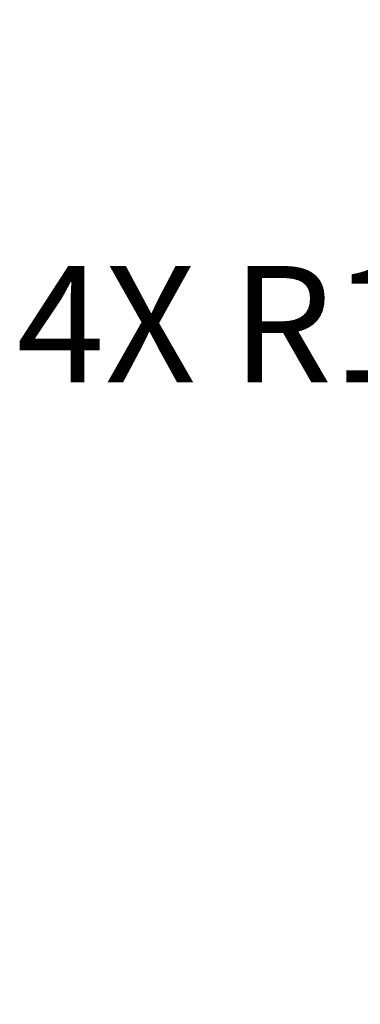
# Model space of a CAD drawing. Units: millimetres. Extents: x 130 to 1021, y 147 to 699.
# Tile 15 of 40: x 195 to 254, y 440 to 610. Entities that reach past the tile are written whole.
import ezdxf

# ---------------------------------------------------------------- set-up
doc = ezdxf.new("R2010")
doc.units = ezdxf.units.MM
doc.header["$MEASUREMENT"] = 0
doc.layers.add('A-ANNO-DIMS', color=2, linetype='Continuous', lineweight=18)
doc.styles.get("Standard").update_dxf_attribs({"font": 'arial.ttf'})
doc.dimstyles.get("Standard").update_dxf_attribs({"dimtxt": 20, "dimasz": 10, "dimexe": 10, "dimexo": 10, "dimgap": 5, "dimtad": 0, "dimtih": 1, "dimtoh": 1, "dimdec": 0, "dimzin": 0, "dimdsep": 46, "dimtxsty": 'Standard', "dimcen": 5, "dimadec": 0, "dimazin": 0, "dimtfac": 1, "dimtdec": 0, "dimtofl": 0, "dimtmove": 0, "dimatfit": 3, "dimfxl": 1, "dimtolj": 1, "dimtzin": 0, "dimarcsym": 0})

# ---------------------------------------------------------------- blocks, each defined once
blk = doc.blocks.new('*D12')
at = {"layer": 'A-ANNO-DIMS', "color": 0, "lineweight": -2, "transparency": 16777216}
for p, q in [((477.37, 661.95), (265.07, 661.95)), ((275.07, 651.95), (275.07, 438.2)), ((275.07, 194.04), (275.07, 407.78)), ((357.16, 184.04), (265.07, 184.04))]:
    blk.add_line(p, q, dxfattribs=at)
at = {"layer": 'A-ANNO-DIMS', "color": 0, "transparency": 16777216}
for points in [[(273.41, 651.95), (276.74, 651.95), (275.07, 661.95)], [(273.41, 194.04), (276.74, 194.04), (275.07, 184.04)]]:
    blk.add_solid(points, dxfattribs=at)
at = {"layer": 'Defpoints', "color": 0, "transparency": 16777216}
for p in [(275.07, 661.95), (487.37, 661.95), (367.16, 184.04)]:
    blk.add_point(p, dxfattribs=at)
at = {"layer": 'A-ANNO-DIMS', "color": 0, "transparency": 16777216, "insert": (275.07, 422.99), "char_height": 20, "attachment_point": 5}
blk.add_mtext('\\A1;477.9', dxfattribs=at)
blk = doc.blocks.new('*D64')
at = {"layer": 'A-ANNO-DIMS', "color": 0, "lineweight": -2, "transparency": 16777216}
for p, q in [((502.05, 450.93), (502.05, 460.93)), ((497.05, 455.93), (507.05, 455.93)), ((363.96, 263.06), (409.92, 327.25)), ((353.96, 263.06), (363.96, 263.06))]:
    blk.add_line(p, q, dxfattribs=at)
at = {"layer": 'A-ANNO-DIMS', "color": 0, "transparency": 16777216}
blk.add_solid([(408.57, 328.22), (411.28, 326.28), (415.74, 335.39)], dxfattribs=at)
at = {"layer": 'Defpoints', "color": 0, "transparency": 16777216}
for p in [(502.05, 455.93), (415.74, 335.39)]:
    blk.add_point(p, dxfattribs=at)
at = {"layer": 'A-ANNO-DIMS', "color": 0, "transparency": 16777216, "insert": (297.8, 263.06), "char_height": 20, "attachment_point": 5}
blk.add_mtext('\\A1;R148.25', dxfattribs=at)
blk = doc.blocks.new('*D66')
at = {"layer": 'A-ANNO-DIMS', "color": 0, "lineweight": -2, "transparency": 16777216}
for p, q in [((341.58, 557.19), (351.58, 557.19)), ((351.58, 557.19), (376.95, 478.14)), ((427.37, 315.98), (427.37, 325.98)), ((422.37, 320.98), (432.37, 320.98))]:
    blk.add_line(p, q, dxfattribs=at)
at = {"layer": 'A-ANNO-DIMS', "color": 0, "transparency": 16777216}
blk.add_solid([(378.53, 478.64), (375.36, 477.63), (380, 468.61)], dxfattribs=at)
at = {"layer": 'Defpoints', "color": 0, "transparency": 16777216}
for p in [(380, 468.61), (427.37, 320.98)]:
    blk.add_point(p, dxfattribs=at)
at = {"layer": 'A-ANNO-DIMS', "color": 0, "transparency": 16777216, "insert": (263.53, 557.19), "char_height": 20, "attachment_point": 5}
blk.add_mtext('\\A1;4X R155.05', dxfattribs=at)

msp = doc.modelspace()

# ---------------------------------------------------------------- dimensions: what is measured, and where the dimension line sits
at = {"layer": 'A-ANNO-DIMS'}
dim = msp.add_linear_dim(base=(275.0738, 661.9473), p1=(367.163, 184.0395), p2=(487.3738, 661.9473), angle=90, dimstyle='Standard', override={"dimdec": 1, "dimlfac": 1, "dimrnd": 0, "dimzin": 0, "dimdsep": 46, "dimlunit": 2}, dxfattribs=at)
dim.commit()
dim.dimension.update_dxf_attribs({"geometry": '*D12', "text_midpoint": (275.0738, 422.9934)})
dim = msp.add_radius_dim(center=(427.3738, 320.9781), mpoint=(380.0022, 468.6132), text='4X <>', dimstyle='Standard', override={"dimdec": 2, "dimlfac": 1, "dimrnd": 0, "dimzin": 0, "dimdsep": 46, "dimlunit": 2}, dxfattribs=at)
dim.commit()
dim.dimension.update_dxf_attribs({"geometry": '*D66', "text_midpoint": (263.5301, 557.1943), "dimtype": 164})
dim = msp.add_radius_dim(center=(502.0489, 455.9263), mpoint=(415.7433, 335.3854), dimstyle='Standard', override={"dimdec": 2, "dimlfac": 1, "dimrnd": 0, "dimzin": 0, "dimdsep": 46, "dimlunit": 2}, dxfattribs=at)
dim.commit()
dim.dimension.update_dxf_attribs({"geometry": '*D64', "text_midpoint": (297.8003, 263.0608), "dimtype": 164})

doc.saveas('drawing.dxf')
